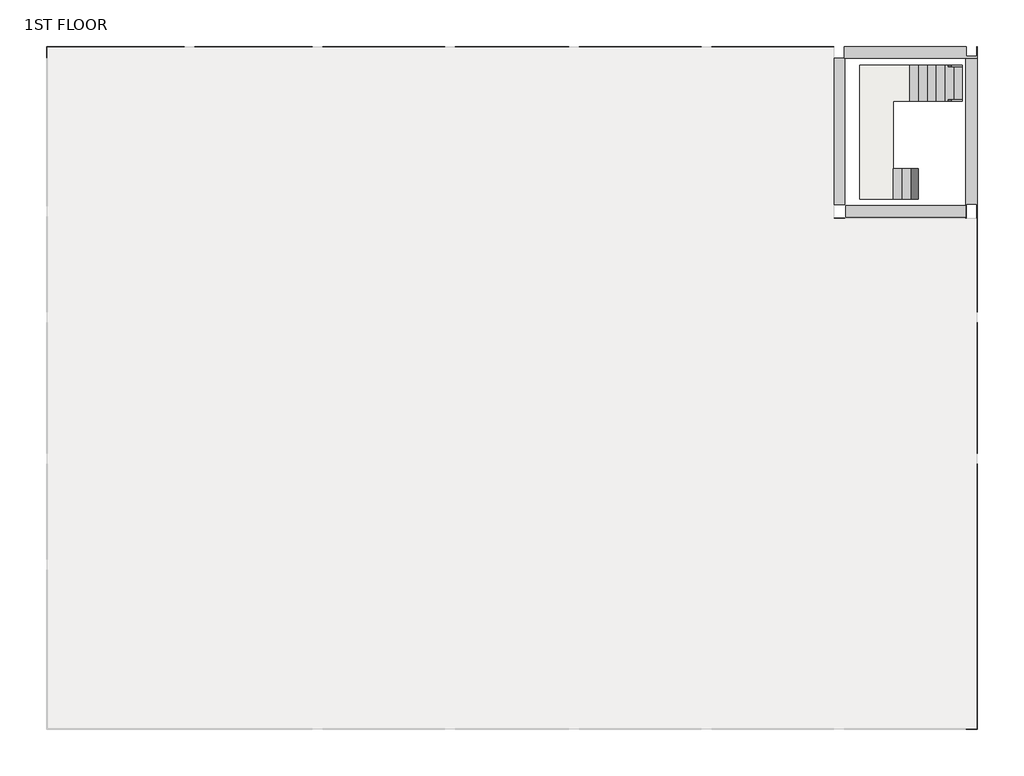
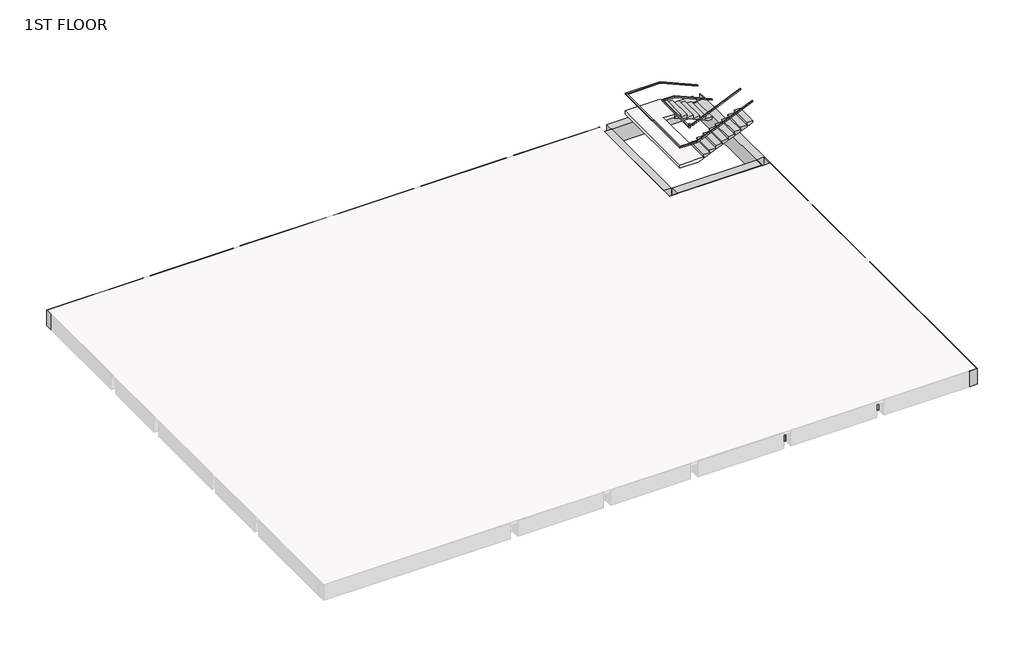
# One storey, part 2 of 2: 5 beams, 2 railings, 2 stair flights, 1 slab.
"""IFC4 building model written with IfcOpenShell, lengths in millimetres."""

from ifc_helpers import new_model, si_unit, frame, origin, place, context, project, spatial, polyline, outline, extrude, faceted_brep, element, save

model = new_model("IFC4")

# Units and contexts
model_context = context("Model", 3, world=origin())
ifc_project = project(units=[si_unit("LENGTHUNIT", "METRE", prefix="MILLI")], contexts=[model_context])

# Site, building, storey
site = spatial("IfcSite", under=ifc_project)
building = spatial("IfcBuilding", under=site)
storey = spatial("IfcBuildingStorey", under=building, Name="1ST FLOOR", Elevation=4572.0)

# Beams
placement = place(None, origin())
element("IfcBeam", 1, ObjectType="M_Concrete-Rectangular Beam : 400 x 800mm", at=placement, inside=storey, context=model_context, shape_type="Brep", body=[
    faceted_brep([(6397.6508981, 16716.9690835, 4572.0), (6397.6508981, 17116.9690835, 4572.0), (6375.4508981, 17116.9690835, 4572.0), (6375.4508981, 16789.9690835, 4572.0), (6019.8508981, 16789.9690835, 4572.0), (6019.8508981, 17116.9690835, 4572.0), (1803.4508981, 17116.9690835, 4572.0), (1803.4508981, 16716.9690835, 4572.0), (1825.6508981, 16716.9690835, 4572.0), (5997.6508981, 16716.9690835, 4572.0), (6397.6508981, 16716.9690835, 3772.0), (1803.4508981, 16716.9690835, 3772.0), (1825.6508981, 16716.9690835, 3772.0), (5997.6508981, 16716.9690835, 3772.0), (6397.6508981, 17116.9690835, 3772.0), (1803.4508981, 17116.9690835, 3772.0), (6019.8508981, 17116.9690835, 3772.0), (6019.8508981, 16789.9690835, 3772.0), (6375.4508981, 16789.9690835, 3772.0), (6375.4508981, 17116.9690835, 3772.0)], [[[0, 1, 2, 3, 4, 5, 6, 7, 8, 9]], [[10, 0, 9, 8, 7, 11, 12, 13]], [[14, 10, 13, 12, 11, 15, 16, 17, 18, 19]], [[1, 14, 19, 2]], [[1, 0, 10, 14]], [[18, 3, 2, 19]], [[3, 18, 17, 4]], [[4, 17, 16, 5]], [[5, 16, 15, 6]], [[7, 6, 15, 11]]]),
    faceted_brep([(-25701.5491019, 16716.9690835, 4572.0), (-25701.5491019, 17116.9690835, 4572.0), (-25701.5491019, 17116.9690835, 3772.0), (-25701.5491019, 16716.9690835, 3772.0), (-25323.7491019, 17094.7690835, 3772.0), (-25323.7491019, 16739.1690835, 3772.0), (-25323.7491019, 16739.1690835, 4419.6), (-25323.7491019, 17094.7690835, 4419.6), (-25679.3491019, 16739.1690835, 3772.0), (-25679.3491019, 16739.1690835, 4419.6), (-25679.3491019, 16716.9690835, 4572.0), (-25679.3491019, 16716.9690835, 4419.6), (-25679.3491019, 17094.7690835, 3772.0), (-25679.3491019, 17094.7690835, 4419.6), (-25679.3491019, 17094.7690835, 4572.0), (-20954.9491019, 16716.9690835, 3772.0), (-20954.9491019, 17116.9690835, 3772.0), (-20954.9491019, 17116.9690835, 4572.0), (-20954.9491019, 17094.7690835, 4572.0), (-20954.9491019, 17094.7690835, 4419.6), (-20954.9491019, 16716.9690835, 4419.6), (-25301.5491019, 16716.9690835, 3772.0), (-20977.1491019, 16716.9690835, 3772.0), (-20977.1491019, 16716.9690835, 4419.6), (-25301.5491019, 16716.9690835, 4419.6)], [[[0, 1, 2, 3]], [[4, 5, 6, 7]], [[5, 8, 9, 6]], [[10, 11, 9, 8, 12, 13, 14]], [[15, 16, 17, 18, 19, 20]], [[1, 0, 10, 14, 18, 17]], [[0, 3, 21, 22, 15, 20, 23, 24, 11, 10]], [[3, 2, 16, 15, 22, 21], [5, 4, 12, 8]], [[2, 1, 17, 16]], [[14, 13, 12, 4, 7, 19, 18]], [[19, 7, 6, 9, 11, 24, 23, 20]]]),
    faceted_brep([(-2768.5491019, 17094.7690835, 4419.6), (1447.8508981, 17094.7690835, 4419.6), (1447.8508981, 17094.7690835, 4572.0), (-2768.5491019, 17094.7690835, 4572.0), (-2768.5491019, 17116.9690835, 3772.0), (-2768.5491019, 16716.9690835, 3772.0), (-2768.5491019, 16716.9690835, 4419.6), (-2768.5491019, 17116.9690835, 4572.0), (1447.8508981, 16716.9690835, 3772.0), (1447.8508981, 17116.9690835, 3772.0), (1447.8508981, 17116.9690835, 4572.0), (1447.8508981, 16716.9690835, 4419.6), (-2746.3491019, 16716.9690835, 3772.0), (1425.6508981, 16716.9690835, 3772.0), (1425.6508981, 16716.9690835, 4419.6), (-2746.3491019, 16716.9690835, 4419.6)], [[[0, 1, 2, 3]], [[4, 5, 6, 0, 3, 7]], [[8, 9, 10, 2, 1, 11]], [[10, 7, 3, 2]], [[5, 12, 13, 8, 11, 14, 15, 6]], [[5, 4, 9, 8, 13, 12]], [[4, 7, 10, 9]], [[1, 0, 6, 15, 14, 11]]]),
    faceted_brep([(-16179.7491019, 17116.9690835, 3772.0), (-16179.7491019, 16716.9690835, 3772.0), (-16179.7491019, 16716.9690835, 4419.6), (-16179.7491019, 17094.7690835, 4419.6), (-16179.7491019, 17094.7690835, 4572.0), (-16179.7491019, 17116.9690835, 4572.0), (-11963.3491019, 16716.9690835, 3772.0), (-11963.3491019, 17116.9690835, 3772.0), (-11963.3491019, 17116.9690835, 4572.0), (-11963.3491019, 17094.7690835, 4572.0), (-11963.3491019, 17094.7690835, 4419.6), (-11963.3491019, 16716.9690835, 4419.6), (-16157.5491019, 16716.9690835, 3772.0), (-11985.5491019, 16716.9690835, 3772.0), (-11985.5491019, 16716.9690835, 4419.6), (-16157.5491019, 16716.9690835, 4419.6)], [[[0, 1, 2, 3, 4, 5]], [[6, 7, 8, 9, 10, 11]], [[8, 5, 4, 9]], [[1, 12, 13, 6, 11, 14, 15, 2]], [[1, 0, 7, 6, 13, 12]], [[0, 5, 8, 7]], [[3, 10, 9, 4]], [[10, 3, 2, 15, 14, 11]]]),
    faceted_brep([(-16535.3491019, 16716.9690835, 3772.0), (-16535.3491019, 17116.9690835, 3772.0), (-16535.3491019, 17116.9690835, 4572.0), (-16535.3491019, 17094.7690835, 4572.0), (-16535.3491019, 17094.7690835, 4419.6), (-16535.3491019, 16716.9690835, 4419.6), (-20599.3491019, 17116.9690835, 4572.0), (-20599.3491019, 17094.7690835, 4572.0), (-20599.3491019, 16716.9690835, 3772.0), (-20577.1491019, 16716.9690835, 3772.0), (-16557.5491019, 16716.9690835, 3772.0), (-16557.5491019, 16716.9690835, 4419.6), (-20577.1491019, 16716.9690835, 4419.6), (-20599.3491019, 16716.9690835, 4419.6), (-20599.3491019, 17116.9690835, 3772.0), (-20599.3491019, 17094.7690835, 4419.6)], [[[0, 1, 2, 3, 4, 5]], [[2, 6, 7, 3]], [[8, 9, 10, 0, 5, 11, 12, 13]], [[1, 0, 10, 9, 8, 14]], [[2, 1, 14, 6]], [[14, 8, 13, 15, 7, 6]], [[15, 4, 3, 7]], [[4, 15, 13, 12, 11, 5]]]),
    faceted_brep([(-11607.7491019, 17116.9690835, 3772.0), (-11607.7491019, 16716.9690835, 3772.0), (-11607.7491019, 16716.9690835, 4419.6), (-11607.7491019, 17094.7690835, 4419.6), (-11607.7491019, 17094.7690835, 4572.0), (-11607.7491019, 17116.9690835, 4572.0), (-7696.1491019, 16716.9690835, 3772.0), (-7696.1491019, 17116.9690835, 3772.0), (-7696.1491019, 17116.9690835, 4572.0), (-7696.1491019, 17094.7690835, 4572.0), (-7696.1491019, 17094.7690835, 4419.6), (-7696.1491019, 16716.9690835, 4419.6), (-11585.5491019, 16716.9690835, 3772.0), (-7718.3491019, 16716.9690835, 3772.0), (-7718.3491019, 16716.9690835, 4419.6), (-11585.5491019, 16716.9690835, 4419.6)], [[[0, 1, 2, 3, 4, 5]], [[6, 7, 8, 9, 10, 11]], [[8, 5, 4, 9]], [[1, 12, 13, 6, 11, 14, 15, 2]], [[1, 0, 7, 6, 13, 12]], [[0, 5, 8, 7]], [[3, 10, 9, 4]], [[10, 3, 2, 15, 14, 11]]]),
    faceted_brep([(-7340.5491019, 17116.9690835, 3772.0), (-7340.5491019, 16716.9690835, 3772.0), (-7340.5491019, 16716.9690835, 4419.6), (-7340.5491019, 17094.7690835, 4419.6), (-7340.5491019, 17094.7690835, 4572.0), (-7340.5491019, 17116.9690835, 4572.0), (-3124.1491019, 16716.9690835, 3772.0), (-3124.1491019, 17116.9690835, 3772.0), (-3124.1491019, 17116.9690835, 4572.0), (-3124.1491019, 17094.7690835, 4572.0), (-3124.1491019, 17094.7690835, 4419.6), (-3124.1491019, 16716.9690835, 4419.6), (-7318.3491019, 16716.9690835, 3772.0), (-3146.3491019, 16716.9690835, 3772.0), (-3146.3491019, 16716.9690835, 4419.6), (-7318.3491019, 16716.9690835, 4419.6)], [[[0, 1, 2, 3, 4, 5]], [[6, 7, 8, 9, 10, 11]], [[8, 5, 4, 9]], [[1, 12, 13, 6, 11, 14, 15, 2]], [[1, 0, 7, 6, 13, 12]], [[0, 5, 8, 7]], [[3, 10, 9, 4]], [[10, 3, 2, 15, 14, 11]]]),
])
element("IfcBeam", 2, ObjectType="M_Concrete-Rectangular Beam : 400 x 800mm", at=placement, inside=storey, context=model_context, shape_type="Brep", body=[
    faceted_brep([(5997.6508981, -6447.8309165, 4572.0), (6397.6508981, -6447.8309165, 4572.0), (6397.6508981, 2718.3690835, 4572.0), (6375.4508981, 2718.3690835, 4572.0), (6375.4508981, -6425.6309165, 4572.0), (5997.6508981, -6425.6309165, 4572.0), (5997.6508981, -6447.8309165, 3772.0), (5997.6508981, -6425.6309165, 4419.6), (5997.6508981, -6047.8309165, 4419.6), (5997.6508981, -961.4309165, 4419.6), (5997.6508981, -561.4309165, 4419.6), (5997.6508981, 2696.1690835, 4419.6), (5997.6508981, 2718.3690835, 4419.6), (5997.6508981, 2718.3690835, 3772.0), (5997.6508981, 2696.1690835, 3772.0), (5997.6508981, -561.4309165, 3772.0), (5997.6508981, -961.4309165, 3772.0), (5997.6508981, -6047.8309165, 3772.0), (6397.6508981, -6447.8309165, 3772.0), (6397.6508981, 2718.3690835, 3772.0), (6375.4508981, -6425.6309165, 3772.0), (6375.4508981, -6070.0309165, 3772.0), (6019.8508981, -6070.0309165, 3772.0), (6019.8508981, -6425.6309165, 3772.0), (6375.4508981, -1015.4309165, 3772.0), (6375.4508981, -507.4309165, 3772.0), (6019.8508981, -507.4309165, 3772.0), (6019.8508981, -1015.4309165, 3772.0), (6375.4508981, 2718.3690835, 4419.6), (6375.4508981, -507.4309165, 4419.6), (6375.4508981, -1015.4309165, 4419.6), (6375.4508981, -6070.0309165, 4419.6), (6375.4508981, -6425.6309165, 4419.6), (6019.8508981, -6425.6309165, 4419.6), (6019.8508981, -6070.0309165, 4419.6), (6019.8508981, -1015.4309165, 4419.6), (6019.8508981, -507.4309165, 4419.6)], [[[0, 1, 2, 3, 4, 5]], [[6, 0, 5, 7, 8, 9, 10, 11, 12, 13, 14, 15, 16, 17]], [[18, 6, 17, 16, 15, 14, 13, 19], [20, 21, 22, 23], [24, 25, 26, 27]], [[1, 18, 19, 2]], [[1, 0, 6, 18]], [[3, 28, 29, 25, 24, 30, 31, 21, 20, 32, 4]], [[4, 32, 20, 23, 33, 7, 5]], [[23, 22, 34, 33]], [[22, 21, 31, 34]], [[19, 13, 12, 28, 3, 2]], [[24, 27, 35, 30]], [[27, 26, 36, 35]], [[26, 25, 29, 36]], [[31, 30, 35, 36, 29, 28, 12, 11, 10, 9, 8, 7, 33, 34]]]),
    faceted_brep([(5997.6508981, 16716.9690835, 3772.0), (5997.6508981, 16716.9690835, 4572.0), (6397.6508981, 16716.9690835, 4572.0), (6397.6508981, 16716.9690835, 3772.0), (5997.6508981, 7950.7690835, 3772.0), (6397.6508981, 7950.7690835, 3772.0), (6397.6508981, 7950.7690835, 4572.0), (6375.4508981, 7950.7690835, 4572.0), (6375.4508981, 7950.7690835, 4419.6), (5997.6508981, 7950.7690835, 4419.6), (5997.6508981, 11630.5690835, 4572.0), (5997.6508981, 11230.5690835, 4572.0), (5997.6508981, 11176.5690835, 4572.0), (6019.8508981, 11176.5690835, 4572.0), (6019.8508981, 11684.5690835, 4572.0), (6375.4508981, 11684.5690835, 4572.0), (6375.4508981, 11176.5690835, 4572.0), (5997.6508981, 11630.5690835, 3772.0), (5997.6508981, 11230.5690835, 3772.0), (5997.6508981, 7972.9690835, 3772.0), (5997.6508981, 7972.9690835, 4419.6), (5997.6508981, 11176.5690835, 4419.6), (6375.4508981, 11176.5690835, 3772.0), (6375.4508981, 11684.5690835, 3772.0), (6019.8508981, 11684.5690835, 3772.0), (6019.8508981, 11176.5690835, 3772.0), (6019.8508981, 11176.5690835, 4419.6), (6375.4508981, 11176.5690835, 4419.6)], [[[0, 1, 2, 3]], [[4, 5, 6, 7, 8, 9]], [[2, 1, 10, 11, 12, 13, 14, 15, 16, 7, 6]], [[1, 0, 17, 18, 19, 4, 9, 20, 21, 12, 11, 10]], [[0, 3, 5, 4, 19, 18, 17], [22, 23, 24, 25]], [[3, 2, 6, 5]], [[22, 25, 26, 27]], [[24, 14, 13, 26, 25]], [[14, 24, 23, 15]], [[8, 27, 26, 21, 20, 9]], [[27, 8, 7, 16, 15, 23, 22]], [[21, 26, 13, 12]]]),
    faceted_brep([(6397.6508981, 7595.1690835, 3772.0), (5997.6508981, 7595.1690835, 3772.0), (5997.6508981, 7595.1690835, 4419.6), (6375.4508981, 7595.1690835, 4419.6), (6375.4508981, 7595.1690835, 4572.0), (6397.6508981, 7595.1690835, 4572.0), (5997.6508981, 3073.9690835, 3772.0), (6397.6508981, 3073.9690835, 3772.0), (6397.6508981, 3073.9690835, 4572.0), (6375.4508981, 3073.9690835, 4572.0), (6375.4508981, 3073.9690835, 4419.6), (5997.6508981, 3073.9690835, 4419.6), (5997.6508981, 7572.9690835, 3772.0), (5997.6508981, 3096.1690835, 3772.0), (5997.6508981, 3096.1690835, 4419.6), (5997.6508981, 7572.9690835, 4419.6)], [[[0, 1, 2, 3, 4, 5]], [[6, 7, 8, 9, 10, 11]], [[8, 5, 4, 9]], [[1, 12, 13, 6, 11, 14, 15, 2]], [[1, 0, 7, 6, 13, 12]], [[0, 5, 8, 7]], [[3, 10, 9, 4]], [[10, 3, 2, 15, 14, 11]]]),
])
element("IfcBeam", 3, ObjectType="M_Concrete-Rectangular Beam : 400 x 800mm", at=placement, inside=storey, context=model_context, shape_type="SweptSolid", body=[
    extrude(outline(polyline([(-2746.3491019, -6047.8309165), (-2768.5491019, -6047.8309165), (-2768.5491019, -6019.2309165), (-3124.1491019, -6019.2309165), (-3124.1491019, -6047.8309165), (-3146.3491019, -6047.8309165), (-3146.3491019, -990.0309165), (-2746.3491019, -990.0309165), (-2746.3491019, -6047.8309165)])), frame((0.0, 0.0, 3772.0), z_axis=(0.0, 0.0, 1.0), x_axis=(1.0, 0.0, 0.0)), (0.0, 0.0, 1.0), 647.6),
    extrude(outline(polyline([(-2768.5491019, 16716.9690835), (-2746.3491019, 16716.9690835), (-2746.3491019, 11659.1690835), (-3146.3491019, 11659.1690835), (-3146.3491019, 16716.9690835), (-3124.1491019, 16716.9690835), (-3124.1491019, 16688.3690835), (-2768.5491019, 16688.3690835), (-2768.5491019, 16716.9690835)])), frame((0.0, 0.0, 3772.0), z_axis=(0.0, 0.0, 1.0), x_axis=(1.0, 0.0, 0.0)), (0.0, 0.0, 1.0), 647.6),
    extrude(outline(polyline([(-3146.3491019, 11201.9690835), (-2746.3491019, 11201.9690835), (-2746.3491019, 8001.5690835), (-3146.3491019, 8001.5690835), (-3146.3491019, 11201.9690835)])), frame((0.0, 0.0, 3772.0), z_axis=(0.0, 0.0, 1.0), x_axis=(1.0, 0.0, 0.0)), (0.0, 0.0, 1.0), 647.6),
    extrude(outline(polyline([(-3146.3491019, 7544.3690835), (-2746.3491019, 7544.3690835), (-2746.3491019, 3124.7690835), (-3146.3491019, 3124.7690835), (-3146.3491019, 7544.3690835)])), frame((0.0, 0.0, 3772.0), z_axis=(0.0, 0.0, 1.0), x_axis=(1.0, 0.0, 0.0)), (0.0, 0.0, 1.0), 647.6),
    extrude(outline(polyline([(-2746.3491019, -532.8309165), (-3146.3491019, -532.8309165), (-3146.3491019, 2667.5690835), (-2746.3491019, 2667.5690835), (-2746.3491019, -532.8309165)])), frame((0.0, 0.0, 3772.0), z_axis=(0.0, 0.0, 1.0), x_axis=(1.0, 0.0, 0.0)), (0.0, 0.0, 1.0), 647.6),
])
element("IfcBeam", 4, ObjectType="M_Concrete-Rectangular Beam : 400 x 800mm", at=placement, inside=storey, context=model_context, shape_type="Brep", body=[
    faceted_brep([(1425.6508981, -990.0309165, 3772.0), (1425.6508981, -6047.8309165, 3772.0), (1425.6508981, -6047.8309165, 4419.6), (1425.6508981, -990.0309165, 4419.6), (1825.6508981, -6047.8309165, 3772.0), (1803.4508981, -6047.8309165, 3772.0), (1803.4508981, -6019.2309165, 3772.0), (1447.8508981, -6019.2309165, 3772.0), (1447.8508981, -6047.8309165, 3772.0), (1825.6508981, -990.0309165, 3772.0), (1825.6508981, -990.0309165, 4419.6), (1825.6508981, -6047.8309165, 4419.6), (1447.8508981, -6047.8309165, 4419.6), (1803.4508981, -6047.8309165, 4419.6), (1803.4508981, -6019.2309165, 4419.6), (1447.8508981, -6019.2309165, 4419.6)], [[[0, 1, 2, 3]], [[4, 5, 6, 7, 8, 1, 0, 9]], [[4, 9, 10, 11]], [[1, 8, 12, 2]], [[6, 5, 13, 14]], [[8, 7, 15, 12]], [[7, 6, 14, 15]], [[5, 4, 11, 13]], [[9, 0, 3, 10]], [[3, 2, 12, 15, 14, 13, 11, 10]]]),
    faceted_brep([(1825.6508981, 16716.9690835, 4572.0), (1825.6508981, 16716.9690835, 3772.0), (1803.4508981, 16716.9690835, 3772.0), (1803.4508981, 16716.9690835, 4572.0), (1803.4508981, 16713.7690835, 3772.0), (1803.4508981, 16713.7690835, 4572.0), (1447.8508981, 16713.7690835, 3772.0), (1447.8508981, 16713.7690835, 4419.6), (1447.8508981, 16713.7690835, 4572.0), (1447.8508981, 16716.9690835, 3772.0), (1447.8508981, 16716.9690835, 4419.6), (1425.6508981, 16716.9690835, 3772.0), (1425.6508981, 16716.9690835, 4419.6), (1425.6508981, 11659.1690835, 3772.0), (1825.6508981, 11659.1690835, 3772.0), (1825.6508981, 11659.1690835, 4572.0), (1447.8508981, 11659.1690835, 4572.0), (1447.8508981, 11659.1690835, 4419.6), (1425.6508981, 11659.1690835, 4419.6)], [[[0, 1, 2, 3]], [[4, 5, 3, 2]], [[5, 4, 6, 7, 8]], [[6, 9, 10, 7]], [[9, 11, 12, 10]], [[13, 14, 15, 16, 17, 18]], [[0, 3, 5, 8, 16, 15]], [[11, 13, 18, 12]], [[2, 1, 14, 13, 11, 9, 6, 4]], [[1, 0, 15, 14]], [[17, 7, 10, 12, 18]], [[7, 17, 16, 8]]]),
    faceted_brep([(1825.6508981, 11201.9690835, 3772.0), (1425.6508981, 11201.9690835, 3772.0), (1425.6508981, 11201.9690835, 4419.6), (1447.8508981, 11201.9690835, 4419.6), (1447.8508981, 11201.9690835, 4572.0), (1825.6508981, 11201.9690835, 4572.0), (1425.6508981, 8001.5690835, 3772.0), (1825.6508981, 8001.5690835, 3772.0), (1825.6508981, 8001.5690835, 4419.6), (1425.6508981, 8001.5690835, 4419.6), (1447.8508981, 11176.5690835, 4572.0), (1825.6508981, 11176.5690835, 4572.0), (1825.6508981, 11176.5690835, 4419.6), (1447.8508981, 11176.5690835, 4419.6)], [[[0, 1, 2, 3, 4, 5]], [[6, 7, 8, 9]], [[5, 4, 10, 11]], [[1, 6, 9, 2]], [[1, 0, 7, 6]], [[0, 5, 11, 12, 8, 7]], [[12, 13, 3, 2, 9, 8]], [[13, 10, 4, 3]], [[10, 13, 12, 11]]]),
    faceted_brep([(1825.6508981, 7544.3690835, 3772.0), (1425.6508981, 7544.3690835, 3772.0), (1425.6508981, 7544.3690835, 4419.6), (1825.6508981, 7544.3690835, 4419.6), (1425.6508981, 3124.7690835, 3772.0), (1825.6508981, 3124.7690835, 3772.0), (1825.6508981, 3124.7690835, 4419.6), (1425.6508981, 3124.7690835, 4419.6)], [[[0, 1, 2, 3]], [[4, 5, 6, 7]], [[1, 4, 7, 2]], [[1, 0, 5, 4]], [[5, 0, 3, 6]], [[3, 2, 7, 6]]]),
    faceted_brep([(1425.6508981, -532.8309165, 3772.0), (1825.6508981, -532.8309165, 3772.0), (1825.6508981, -532.8309165, 4419.6), (1425.6508981, -532.8309165, 4419.6), (1425.6508981, 2667.5690835, 3772.0), (1425.6508981, 2667.5690835, 4419.6), (1825.6508981, 2667.5690835, 3772.0), (1825.6508981, 2667.5690835, 4419.6)], [[[0, 1, 2, 3]], [[4, 0, 3, 5]], [[1, 0, 4, 6]], [[1, 6, 7, 2]], [[6, 4, 5, 7]], [[3, 2, 7, 5]]]),
])
element("IfcBeam", 5, ObjectType="M_Concrete-Rectangular Beam : 400 x 800mm", at=placement, inside=storey, context=model_context, shape_type="SweptSolid", body=[
    extrude(outline(polyline([(-25301.5491019, 11608.3690835), (-25301.5491019, 11630.5690835), (-21005.7491019, 11630.5690835), (-21005.7491019, 11230.5690835), (-25301.5491019, 11230.5690835), (-25301.5491019, 11252.7690835), (-25247.5491019, 11252.7690835), (-25247.5491019, 11608.3690835), (-25301.5491019, 11608.3690835)])), frame((0.0, 0.0, 3772.0), z_axis=(0.0, 0.0, 1.0), x_axis=(1.0, 0.0, 0.0)), (0.0, 0.0, 1.0), 647.6),
    extrude(outline(polyline([(5997.6508981, 11630.5690835), (5997.6508981, 11230.5690835), (1854.2508981, 11230.5690835), (1854.2508981, 11630.5690835), (5997.6508981, 11630.5690835)])), frame((0.0, 0.0, 3772.0), z_axis=(0.0, 0.0, 1.0), x_axis=(1.0, 0.0, 0.0)), (0.0, 0.0, 1.0), 800.0),
    extrude(outline(polyline([(-20548.5491019, 11230.5690835), (-20548.5491019, 11630.5690835), (-16586.1491019, 11630.5690835), (-16586.1491019, 11230.5690835), (-20548.5491019, 11230.5690835)])), frame((0.0, 0.0, 3772.0), z_axis=(0.0, 0.0, 1.0), x_axis=(1.0, 0.0, 0.0)), (0.0, 0.0, 1.0), 647.6),
    extrude(outline(polyline([(-16128.9491019, 11230.5690835), (-16128.9491019, 11630.5690835), (-12014.1491019, 11630.5690835), (-12014.1491019, 11230.5690835), (-16128.9491019, 11230.5690835)])), frame((0.0, 0.0, 3772.0), z_axis=(0.0, 0.0, 1.0), x_axis=(1.0, 0.0, 0.0)), (0.0, 0.0, 1.0), 647.6),
    extrude(outline(polyline([(-11556.9491019, 11230.5690835), (-11556.9491019, 11630.5690835), (-7746.9491019, 11630.5690835), (-7746.9491019, 11230.5690835), (-11556.9491019, 11230.5690835)])), frame((0.0, 0.0, 3772.0), z_axis=(0.0, 0.0, 1.0), x_axis=(1.0, 0.0, 0.0)), (0.0, 0.0, 1.0), 647.6),
    extrude(outline(polyline([(-7289.7491019, 11230.5690835), (-7289.7491019, 11630.5690835), (-3174.9491019, 11630.5690835), (-3174.9491019, 11230.5690835), (-7289.7491019, 11230.5690835)])), frame((0.0, 0.0, 3772.0), z_axis=(0.0, 0.0, 1.0), x_axis=(1.0, 0.0, 0.0)), (0.0, 0.0, 1.0), 647.6),
    extrude(outline(polyline([(-2717.7491019, 11230.5690835), (-2717.7491019, 11630.5690835), (1397.0508981, 11630.5690835), (1397.0508981, 11230.5690835), (-2717.7491019, 11230.5690835)])), frame((0.0, 0.0, 3772.0), z_axis=(0.0, 0.0, 1.0), x_axis=(1.0, 0.0, 0.0)), (0.0, 0.0, 1.0), 647.6),
])

# Railings
element("IfcRailing", 6, ObjectType="Handrail", at=placement, inside=storey, context=model_context, shape_type="Brep", body=[
    faceted_brep([(5878.2258195, 16426.305974, 5616.575), (5878.2258195, 16426.305974, 5561.3359813), (5878.2258195, 16477.105974, 5561.3359813), (5878.2258195, 16477.105974, 5616.575), (4049.4258195, 16426.305974, 6397.625), (4039.0320197, 16426.305974, 6346.825), (4039.0320197, 16477.105974, 6346.825), (4049.4258195, 16477.105974, 6397.625), (2398.4258195, 16426.305974, 6397.625), (2398.4258195, 16426.305974, 6346.825), (2347.6258195, 16477.105974, 6346.825), (2347.6258195, 16477.105974, 6397.625), (2398.4258195, 11896.1816424, 6397.625), (2398.4258195, 11896.1816424, 6346.825), (2347.6258195, 11845.3816424, 6346.825), (2347.6258195, 11845.3816424, 6397.625), (3188.2923097, 11896.1816424, 6397.625), (3198.6861096, 11896.1816424, 6346.825), (3198.6861096, 11845.3816424, 6346.825), (3188.2923097, 11845.3816424, 6397.625), (5931.4923097, 11896.1816424, 7569.2), (5931.4923097, 11845.3816424, 7569.2), (5931.4923097, 11845.3816424, 7513.9609813), (5931.4923097, 11896.1816424, 7513.9609813)], [[[0, 1, 2, 3]], [[1, 0, 4, 5]], [[2, 1, 5, 6]], [[3, 2, 6, 7]], [[0, 3, 7, 4]], [[5, 4, 8, 9]], [[6, 5, 9, 10]], [[7, 6, 10, 11]], [[4, 7, 11, 8]], [[9, 8, 12, 13]], [[10, 9, 13, 14]], [[11, 10, 14, 15]], [[8, 11, 15, 12]], [[13, 12, 16, 17]], [[14, 13, 17, 18]], [[15, 14, 18, 19]], [[12, 15, 19, 16]], [[20, 21, 22, 23]], [[17, 16, 20, 23]], [[18, 17, 23, 22]], [[19, 18, 22, 21]], [[16, 19, 21, 20]]]),
])
element("IfcRailing", 7, ObjectType="Handrail", at=placement, inside=storey, context=model_context, shape_type="Brep", body=[
    faceted_brep([(5878.2258195, 15223.6852874, 5616.575), (5878.2258195, 15223.6852874, 5561.3359813), (5878.2258195, 15274.4852874, 5561.3359813), (5878.2258195, 15274.4852874, 5616.575), (4049.4258195, 15223.6852874, 6397.625), (4039.0320197, 15223.6852874, 6346.825), (4039.0320197, 15274.4852874, 6346.825), (4049.4258195, 15274.4852874, 6397.625), (3493.0923097, 15223.6852874, 6397.625), (3493.0923097, 15223.6852874, 6346.825), (3442.2923097, 15274.4852874, 6346.825), (3442.2923097, 15274.4852874, 6397.625), (3493.0923097, 12985.9409784, 6397.625), (3493.0923097, 12935.1409784, 6346.825), (3442.2923097, 12935.1409784, 6346.825), (3442.2923097, 12985.9409784, 6397.625), (3493.0923097, 12985.9409784, 6560.34375), (3493.0923097, 12935.1409784, 6509.54375), (3442.2923097, 12935.1409784, 6509.54375), (3442.2923097, 12985.9409784, 6560.34375), (3493.0923097, 12909.7409784, 6560.34375), (3493.0923097, 12909.7409784, 6509.54375), (3442.2923097, 12858.9409784, 6509.54375), (3442.2923097, 12858.9409784, 6560.34375), (3569.2923097, 12909.7409784, 6560.34375), (3579.6861096, 12909.7409784, 6509.54375), (3579.6861096, 12858.9409784, 6509.54375), (3569.2923097, 12858.9409784, 6560.34375), (5931.4923097, 12909.7409784, 7569.2), (5931.4923097, 12858.9409784, 7569.2), (5931.4923097, 12858.9409784, 7513.9609813), (5931.4923097, 12909.7409784, 7513.9609813)], [[[0, 1, 2, 3]], [[1, 0, 4, 5]], [[2, 1, 5, 6]], [[3, 2, 6, 7]], [[0, 3, 7, 4]], [[5, 4, 8, 9]], [[6, 5, 9, 10]], [[7, 6, 10, 11]], [[4, 7, 11, 8]], [[9, 8, 12, 13]], [[10, 9, 13, 14]], [[11, 10, 14, 15]], [[8, 11, 15, 12]], [[13, 12, 16, 17]], [[14, 13, 17, 18]], [[15, 14, 18, 19]], [[12, 15, 19, 16]], [[17, 16, 20, 21]], [[18, 17, 21, 22]], [[19, 18, 22, 23]], [[16, 19, 23, 20]], [[21, 20, 24, 25]], [[22, 21, 25, 26]], [[23, 22, 26, 27]], [[20, 23, 27, 24]], [[28, 29, 30, 31]], [[25, 24, 28, 31]], [[26, 25, 31, 30]], [[27, 26, 30, 29]], [[24, 27, 29, 28]]]),
])

# Slab
element("IfcSlab", 8, ObjectType="7\" Thickness", at=placement, inside=storey, context=model_context, shape_type="Brep", body=[
    faceted_brep([(4049.4258195, 16477.105974, 5483.225), (4049.4258195, 15223.6852874, 5483.225), (4030.3758195, 15223.6852874, 5353.05), (4030.3758195, 16477.105974, 5353.05), (2347.6258195, 16477.105974, 5483.225), (2347.6258195, 11845.3816424, 5483.225), (3257.5052912, 11845.3816424, 5483.225), (3493.0923097, 11845.3816424, 5483.225), (3512.1423097, 11845.3816424, 5483.225), (3512.1423097, 12909.7409784, 5483.225), (3493.0923097, 12909.7409784, 5483.225), (3493.0923097, 15223.6852874, 5483.225), (3980.212838, 15223.6852874, 5483.225), (3980.212838, 16477.105974, 5483.225), (4030.3758195, 15223.6852874, 5284.0012267), (4030.3758195, 16477.105974, 5284.0012267), (3980.212838, 16477.105974, 5305.425), (2347.6258195, 16477.105974, 5305.425), (2347.6258195, 11845.3816424, 5305.425), (3257.5052912, 11845.3816424, 5305.425), (3493.0923097, 11845.3816424, 5406.0402892), (3512.1423097, 11845.3816424, 5414.1762267), (3512.1423097, 12909.7409784, 5414.1762267), (3493.0923097, 12909.7409784, 5406.0402892), (3493.0923097, 12909.7409784, 5305.425), (3493.0923097, 15223.6852874, 5305.425), (3980.212838, 15223.6852874, 5305.425), (3257.5052912, 12909.7409784, 5305.425)], [[[0, 1, 2, 3]], [[4, 5, 6, 7, 8, 9, 10, 11, 12, 1, 0, 13]], [[3, 2, 14, 15]], [[0, 3, 15, 16, 17, 4, 13]], [[5, 4, 17, 18]], [[5, 18, 19, 20, 7, 6]], [[8, 7, 20, 21]], [[9, 8, 21, 22]], [[10, 9, 22, 23]], [[11, 10, 23, 24, 25]], [[2, 1, 12, 11, 25, 26, 14]], [[24, 27, 19, 18, 17, 16, 26, 25]], [[27, 24, 23]], [[26, 16, 15, 14]], [[19, 27, 23, 22, 21, 20]]]),
])

# Stair flights
element("IfcStairFlight", 9, ObjectType="3/4\" Nosing", at=placement, inside=storey, context=model_context, shape_type="Brep", body=[
    faceted_brep([(5878.2258195, 16477.105974, 4702.175), (5878.2258195, 15223.6852874, 4702.175), (5859.1758195, 15223.6852874, 4572.0), (5859.1758195, 16477.105974, 4572.0), (5554.3758195, 16477.105974, 4702.175), (5554.3758195, 15223.6852874, 4702.175), (5554.3758195, 15223.6852874, 4633.1262267), (5697.5006429, 15223.6852874, 4572.0), (5697.5006429, 16477.105974, 4572.0), (5554.3758195, 16477.105974, 4633.1262267), (5573.4258195, 15223.6852874, 4832.35), (5573.4258195, 16477.105974, 4832.35), (5249.5758195, 16477.105974, 4832.35), (5249.5758195, 15223.6852874, 4832.35), (5249.5758195, 15223.6852874, 4763.3012267), (5249.5758195, 16477.105974, 4763.3012267), (5268.6258195, 15223.6852874, 4962.525), (5268.6258195, 16477.105974, 4962.525), (4944.7758195, 16477.105974, 4962.525), (4944.7758195, 15223.6852874, 4962.525), (4944.7758195, 15223.6852874, 4893.4762267), (4944.7758195, 16477.105974, 4893.4762267), (4963.8258195, 15223.6852874, 5092.7), (4963.8258195, 16477.105974, 5092.7), (4639.9758195, 16477.105974, 5092.7), (4639.9758195, 15223.6852874, 5092.7), (4639.9758195, 15223.6852874, 5023.6512267), (4639.9758195, 16477.105974, 5023.6512267), (4659.0258195, 15223.6852874, 5222.875), (4659.0258195, 16477.105974, 5222.875), (4335.1758195, 16477.105974, 5222.875), (4335.1758195, 15223.6852874, 5222.875), (4335.1758195, 15223.6852874, 5153.8262267), (4335.1758195, 16477.105974, 5153.8262267), (4030.3758195, 15223.6852874, 5353.05), (4049.4258195, 15223.6852874, 5353.05), (4354.2258195, 15223.6852874, 5353.05), (4354.2258195, 16477.105974, 5353.05), (4049.4258195, 16477.105974, 5353.05), (4030.3758195, 16477.105974, 5353.05), (4030.3758195, 15223.6852874, 5284.0012267), (4049.4258195, 15223.6852874, 5275.8652892), (4049.4258195, 16477.105974, 5275.8652892), (4030.3758195, 16477.105974, 5284.0012267)], [[[0, 1, 2, 3]], [[1, 0, 4, 5]], [[1, 5, 6, 7, 2]], [[4, 0, 3, 8, 9]], [[10, 11, 12, 13]], [[10, 13, 14, 6, 5]], [[12, 11, 4, 9, 15]], [[5, 4, 11, 10]], [[16, 17, 18, 19]], [[16, 19, 20, 14, 13]], [[18, 17, 12, 15, 21]], [[13, 12, 17, 16]], [[22, 23, 24, 25]], [[22, 25, 26, 20, 19]], [[24, 23, 18, 21, 27]], [[19, 18, 23, 22]], [[28, 29, 30, 31]], [[28, 31, 32, 26, 25]], [[30, 29, 24, 27, 33]], [[25, 24, 29, 28]], [[34, 35, 36, 37, 38, 39]], [[35, 34, 40, 41]], [[38, 37, 30, 33, 42]], [[34, 39, 43, 40]], [[31, 30, 37, 36]], [[3, 2, 7, 8]], [[8, 7, 6, 14, 20, 26, 32, 41, 40, 43, 42, 33, 27, 21, 15, 9]], [[36, 35, 41, 32, 31]], [[39, 38, 42, 43]]]),
])
element("IfcStairFlight", 10, ObjectType="3/4\" Nosing", at=placement, inside=storey, context=model_context, shape_type="Brep", body=[
    faceted_brep([(3493.0923097, 11845.3816424, 5613.4), (3493.0923097, 12909.7409784, 5613.4), (3512.1423097, 12909.7409784, 5483.225), (3512.1423097, 11845.3816424, 5483.225), (3816.9423097, 11845.3816424, 5613.4), (3816.9423097, 12909.7409784, 5613.4), (3816.9423097, 12909.7409784, 5544.3512267), (3512.1423097, 12909.7409784, 5414.1762267), (3512.1423097, 11845.3816424, 5414.1762267), (3816.9423097, 11845.3816424, 5544.3512267), (3797.8923097, 12909.7409784, 5743.575), (3797.8923097, 11845.3816424, 5743.575), (4121.7423097, 11845.3816424, 5743.575), (4121.7423097, 12909.7409784, 5743.575), (4121.7423097, 12909.7409784, 5674.5262267), (4121.7423097, 11845.3816424, 5674.5262267), (4102.6923097, 12909.7409784, 5873.75), (4102.6923097, 11845.3816424, 5873.75), (4426.5423097, 11845.3816424, 5873.75), (4426.5423097, 12909.7409784, 5873.75), (4426.5423097, 12909.7409784, 5804.7012267), (4426.5423097, 11845.3816424, 5804.7012267), (4407.4923097, 12909.7409784, 6003.925), (4407.4923097, 11845.3816424, 6003.925), (4731.3423097, 11845.3816424, 6003.925), (4731.3423097, 12909.7409784, 6003.925), (4731.3423097, 12909.7409784, 5934.8762267), (4731.3423097, 11845.3816424, 5934.8762267), (4712.2923097, 12909.7409784, 6134.1), (4712.2923097, 11845.3816424, 6134.1), (5036.1423097, 11845.3816424, 6134.1), (5036.1423097, 12909.7409784, 6134.1), (5036.1423097, 12909.7409784, 6065.0512267), (5036.1423097, 11845.3816424, 6065.0512267), (5017.0923097, 12909.7409784, 6264.275), (5017.0923097, 11845.3816424, 6264.275), (5340.9423097, 11845.3816424, 6264.275), (5340.9423097, 12909.7409784, 6264.275), (5340.9423097, 12909.7409784, 6195.2262267), (5340.9423097, 11845.3816424, 6195.2262267), (5321.8923097, 12909.7409784, 6394.45), (5321.8923097, 11845.3816424, 6394.45), (5645.7423097, 11845.3816424, 6394.45), (5645.7423097, 12909.7409784, 6394.45), (5645.7423097, 12909.7409784, 6325.4012267), (5645.7423097, 11845.3816424, 6325.4012267), (5626.6923097, 12909.7409784, 6524.625), (5626.6923097, 11845.3816424, 6524.625), (5931.4923097, 11845.3816424, 6524.625), (5931.4923097, 12909.7409784, 6524.625), (5931.4923097, 12909.7409784, 6447.4402892), (5931.4923097, 11845.3816424, 6447.4402892)], [[[0, 1, 2, 3]], [[1, 0, 4, 5]], [[1, 5, 6, 7, 2]], [[3, 2, 7, 8]], [[4, 0, 3, 8, 9]], [[10, 11, 12, 13]], [[10, 13, 14, 6, 5]], [[12, 11, 4, 9, 15]], [[11, 10, 5, 4]], [[16, 17, 18, 19]], [[16, 19, 20, 14, 13]], [[18, 17, 12, 15, 21]], [[17, 16, 13, 12]], [[22, 23, 24, 25]], [[22, 25, 26, 20, 19]], [[24, 23, 18, 21, 27]], [[23, 22, 19, 18]], [[28, 29, 30, 31]], [[28, 31, 32, 26, 25]], [[30, 29, 24, 27, 33]], [[29, 28, 25, 24]], [[34, 35, 36, 37]], [[34, 37, 38, 32, 31]], [[36, 35, 30, 33, 39]], [[35, 34, 31, 30]], [[40, 41, 42, 43]], [[40, 43, 44, 38, 37]], [[42, 41, 36, 39, 45]], [[41, 40, 37, 36]], [[46, 47, 48, 49]], [[46, 49, 50, 44, 43]], [[48, 47, 42, 45, 51]], [[49, 48, 51, 50]], [[47, 46, 43, 42]], [[7, 6, 14, 20, 26, 32, 38, 44, 50, 51, 45, 39, 33, 27, 21, 15, 9, 8]]]),
])

save(model, "model.ifc")

# Revit data of these elements
# Type "M_Concrete-Rectangular Beam : 400 x 800mm"
#   Length [instance default] = 5' - 0"
#   b = 1' - 3.74803"
#   h = 2' - 7.49606"
#   Structural Material [instance default] = Concrete, Cast-in-Place gray
#   Assembly Code = ""
# Type "Handrail"
#   Assembly Code = "C2010400"
#   built-in parameter 1008612 = 0.0416667 (stored number, unit not read)
#   built-in parameter 1008611 = 0.0416667 (stored number, unit not read)
#   built-in parameter 1008609 = 0.333333 (stored number, unit not read)
#   built-in parameter 1008604 = 0.166667 (stored number, unit not read)
#   built-in parameter 1008603 = 0.166667 (stored number, unit not read)
#   Railing Height = 3' - 0"
#   built-in parameter 1008630 = 2
#   built-in parameter 1008610 = 2
#   built-in parameter 1008618 = Baluster - Square : 3/4"
# Elements 1, 2 (IfcBeam, "M_Concrete-Rectangular Beam : 400 x 800mm")
#   Structural Material = Concrete, Cast-in-Place gray
#   Phase Created = New Construction
#   Materials on its faces: "Concrete, Cast-in-Place gray"
# Elements 3, 4, 5 (IfcBeam, "M_Concrete-Rectangular Beam : 400 x 800mm")
#   Comments = ""
#   Structural Material = Concrete, Cast-in-Place gray
#   Phase Created = New Construction
#   Materials on its faces: "Concrete, Cast-in-Place gray"
# Elements 6, 7 (IfcRailing, "Handrail")
#   Phase Created = New Construction
# Element 8 (IfcSlab, "7\" Thickness")
#   Phase Created = New Construction
#   Materials on its faces: "Concrete, Cast-in-Place gray"
# Elements 9, 10 (IfcStairFlight, "3/4\" Nosing")
#   Phase Created = New Construction
#   Materials on its faces: "Concrete, Cast-in-Place gray"
# Materials
#   "Concrete, Cast-in-Place gray": class "Concrete", colour RGB 192 192 192, transparency 0, Description = "Cast-in-place concrete", Cost = 0
